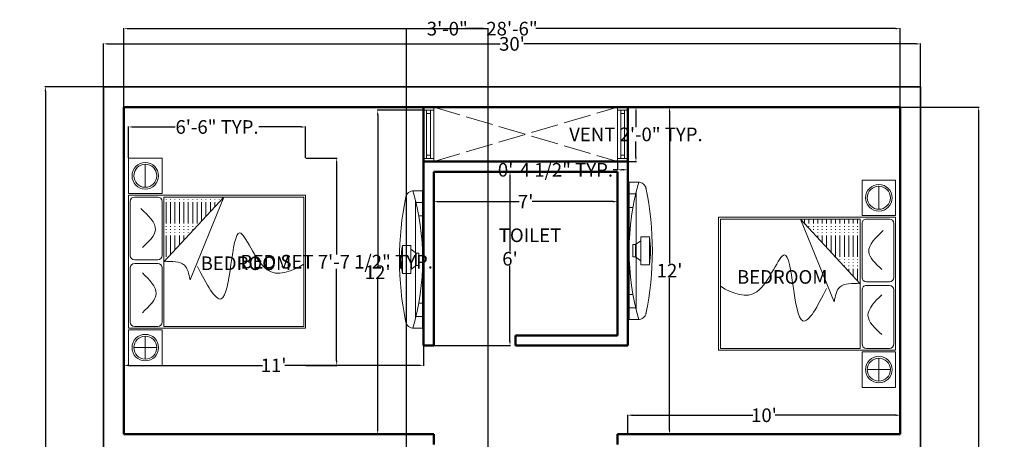
# Model space of a CAD drawing. Units: inches. Extents: x 134 to 568, y 15 to 554.
# Tile 7 of 7: x 134 to 568, y 369 to 554. Entities that reach past the tile are written whole.
import ezdxf

# ---------------------------------------------------------------- set-up
doc = ezdxf.new("R2010")
doc.units = ezdxf.units.IN
doc.header["$MEASUREMENT"] = 0
doc.linetypes.add('ACAD_ISO02W100', pattern=[15, 12, -3])
for name, color, linetype, lineweight in [('A-ANNO-DIMS', 2, 'Continuous', 18), ('A-AREA-IDEN', 7, 'Continuous', 25), ('A-EQPM', 8, 'Continuous', 18), ('A-FLOR-OPEN', 8, 'ACAD_ISO02W100', 18), ('A-FURN', 9, 'Continuous', 18), ('A-GLAZ', 4, 'Continuous', 18), ('A-WALL', 7, 'Continuous', 50), ('C-PROP', 7, 'Continuous', 35)]:
    doc.layers.add(name, color=color, linetype=linetype, lineweight=lineweight)
doc.styles.get("Standard").update_dxf_attribs({"font": 'arial.ttf'})
doc.dimstyles.get("Standard").update_dxf_attribs({"dimtxt": 6, "dimasz": 2, "dimexe": 0.18, "dimexo": 0.0625, "dimgap": 0.09, "dimtad": 0, "dimtih": 1, "dimtoh": 1, "dimdec": 0, "dimzin": 0, "dimdsep": 46, "dimlunit": 4, "dimtxsty": 'Standard', "dimcen": 0.09, "dimadec": 0, "dimazin": 0, "dimtfac": 1, "dimtdec": 0, "dimtofl": 0, "dimtmove": 0, "dimatfit": 3, "dimfxl": 1, "dimtolj": 1, "dimtzin": 0, "dimarcsym": 0})

# ---------------------------------------------------------------- blocks, each defined once
blk = doc.blocks.new('*D1')
at = {"layer": 'A-ANNO-DIMS', "color": 0, "lineweight": -2, "transparency": 16777216}
for p, q in [((171.08, 524.64), (171.08, 543.61)), ((173.08, 543.43), (345.9, 543.43)), ((529.08, 543.43), (356.26, 543.43)), ((531.08, 524.64), (531.08, 543.61))]:
    blk.add_line(p, q, dxfattribs=at)
at = {"layer": 'A-ANNO-DIMS', "color": 0, "transparency": 16777216}
for points in [[(173.08, 543.76), (173.08, 543.1), (171.08, 543.43)], [(529.08, 543.76), (529.08, 543.1), (531.08, 543.43)]]:
    blk.add_solid(points, dxfattribs=at)
at = {"layer": 'Defpoints', "color": 0, "transparency": 16777216}
for p in [(531.08, 543.43), (171.08, 524.58), (531.08, 524.58)]:
    blk.add_point(p, dxfattribs=at)
at = {"layer": 'A-ANNO-DIMS', "color": 0, "transparency": 16777216, "insert": (351.08, 543.43), "char_height": 6, "attachment_point": 5}
blk.add_mtext("\\A1;30'", dxfattribs=at)
blk = doc.blocks.new('*D16')
at = {"layer": 'A-ANNO-DIMS', "color": 0, "lineweight": -2, "transparency": 16777216}
for p, q in [((316.65, 487.08), (350.37, 487.08)), ((350.19, 485.08), (350.19, 451.99)), ((350.19, 412.58), (350.19, 445.68)), ((316.65, 410.58), (350.37, 410.58))]:
    blk.add_line(p, q, dxfattribs=at)
at = {"layer": 'A-ANNO-DIMS', "color": 0, "transparency": 16777216}
for points in [[(349.85, 485.08), (350.52, 485.08), (350.19, 487.08)], [(349.85, 412.58), (350.52, 412.58), (350.19, 410.58)]]:
    blk.add_solid(points, dxfattribs=at)
at = {"layer": 'Defpoints', "color": 0, "transparency": 16777216}
for p in [(316.58, 487.08), (316.58, 410.58), (350.19, 410.58)]:
    blk.add_point(p, dxfattribs=at)
at = {"layer": 'A-ANNO-DIMS', "color": 0, "transparency": 16777216, "insert": (350.19, 448.83), "char_height": 6, "attachment_point": 5}
blk.add_mtext("\\A1;6'", dxfattribs=at)
blk = doc.blocks.new('*D17')
at = {"layer": 'A-ANNO-DIMS', "color": 0, "lineweight": -2, "transparency": 16777216}
for p, q in [((316.58, 487.02), (316.58, 473.78)), ((397.58, 487.02), (397.58, 473.78)), ((318.58, 473.96), (354.26, 473.96)), ((395.58, 473.96), (359.91, 473.96))]:
    blk.add_line(p, q, dxfattribs=at)
at = {"layer": 'A-ANNO-DIMS', "color": 0, "transparency": 16777216}
for points in [[(318.58, 474.29), (318.58, 473.62), (316.58, 473.96)], [(395.58, 474.29), (395.58, 473.62), (397.58, 473.96)]]:
    blk.add_solid(points, dxfattribs=at)
at = {"layer": 'Defpoints', "color": 0, "transparency": 16777216}
for p in [(316.58, 487.08), (397.58, 487.08), (397.58, 473.96)]:
    blk.add_point(p, dxfattribs=at)
at = {"layer": 'A-ANNO-DIMS', "color": 0, "transparency": 16777216, "insert": (357.08, 473.96), "char_height": 6, "attachment_point": 5}
blk.add_mtext("\\A1;7'", dxfattribs=at)
blk = doc.blocks.new('*D18')
at = {"layer": 'A-ANNO-DIMS', "color": 0, "lineweight": -2, "transparency": 16777216}
for p, q in [((312.02, 514.18), (291.74, 514.18)), ((291.92, 512.18), (291.92, 445.98)), ((291.92, 373.58), (291.92, 439.78)), ((316.52, 371.58), (291.74, 371.58))]:
    blk.add_line(p, q, dxfattribs=at)
at = {"layer": 'A-ANNO-DIMS', "color": 0, "transparency": 16777216}
for points in [[(291.59, 512.18), (292.25, 512.18), (291.92, 514.18)], [(291.59, 373.58), (292.25, 373.58), (291.92, 371.58)]]:
    blk.add_solid(points, dxfattribs=at)
at = {"layer": 'Defpoints', "color": 0, "transparency": 16777216}
for p in [(312.08, 514.18), (291.92, 371.58), (316.58, 371.58)]:
    blk.add_point(p, dxfattribs=at)
at = {"layer": 'A-ANNO-DIMS', "color": 0, "transparency": 16777216, "insert": (291.92, 442.88), "char_height": 6, "attachment_point": 5}
blk.add_mtext("\\A1;12'", dxfattribs=at)
blk = doc.blocks.new('*D19')
at = {"layer": 'A-ANNO-DIMS', "color": 0, "lineweight": -2, "transparency": 16777216}
for p, q in [((312.08, 410.52), (312.08, 401.71)), ((180.08, 371.64), (180.08, 402.07)), ((182.08, 401.89), (241.18, 401.89)), ((310.08, 401.89), (250.98, 401.89))]:
    blk.add_line(p, q, dxfattribs=at)
at = {"layer": 'A-ANNO-DIMS', "color": 0, "transparency": 16777216}
for points in [[(182.08, 402.22), (182.08, 401.55), (180.08, 401.89)], [(310.08, 402.22), (310.08, 401.55), (312.08, 401.89)]]:
    blk.add_solid(points, dxfattribs=at)
at = {"layer": 'Defpoints', "color": 0, "transparency": 16777216}
for p in [(312.08, 410.58), (180.08, 401.89), (180.08, 371.58)]:
    blk.add_point(p, dxfattribs=at)
at = {"layer": 'A-ANNO-DIMS', "color": 0, "transparency": 16777216, "insert": (246.08, 401.89), "char_height": 6, "attachment_point": 5}
blk.add_mtext("\\A1;11'", dxfattribs=at)
blk = doc.blocks.new('*D20')
at = {"layer": 'A-ANNO-DIMS', "color": 0, "lineweight": -2, "transparency": 16777216}
for p, q in [((522.02, 515.58), (420.3, 515.58)), ((420.48, 513.58), (420.48, 446.68)), ((420.48, 373.58), (420.48, 440.48)), ((522.02, 371.58), (420.3, 371.58))]:
    blk.add_line(p, q, dxfattribs=at)
at = {"layer": 'A-ANNO-DIMS', "color": 0, "transparency": 16777216}
for points in [[(420.14, 513.58), (420.81, 513.58), (420.48, 515.58)], [(420.14, 373.58), (420.81, 373.58), (420.48, 371.58)]]:
    blk.add_solid(points, dxfattribs=at)
at = {"layer": 'Defpoints', "color": 0, "transparency": 16777216}
for p in [(420.48, 515.58), (522.08, 515.58), (522.08, 371.58)]:
    blk.add_point(p, dxfattribs=at)
at = {"layer": 'A-ANNO-DIMS', "color": 0, "transparency": 16777216, "insert": (420.48, 443.58), "char_height": 6, "attachment_point": 5}
blk.add_mtext("\\A1;12'", dxfattribs=at)
blk = doc.blocks.new('*D21')
at = {"layer": 'A-ANNO-DIMS', "color": 0, "lineweight": -2, "transparency": 16777216}
for p, q in [((402.08, 371.64), (402.08, 380.11)), ((404.08, 379.93), (457.18, 379.93)), ((520.08, 379.93), (466.98, 379.93)), ((522.08, 371.64), (522.08, 380.11))]:
    blk.add_line(p, q, dxfattribs=at)
at = {"layer": 'A-ANNO-DIMS', "color": 0, "transparency": 16777216}
for points in [[(404.08, 380.27), (404.08, 379.6), (402.08, 379.93)], [(520.08, 380.27), (520.08, 379.6), (522.08, 379.93)]]:
    blk.add_solid(points, dxfattribs=at)
at = {"layer": 'Defpoints', "color": 0, "transparency": 16777216}
for p in [(402.08, 379.93), (402.08, 371.58), (522.08, 371.58)]:
    blk.add_point(p, dxfattribs=at)
at = {"layer": 'A-ANNO-DIMS', "color": 0, "transparency": 16777216, "insert": (462.08, 379.93), "char_height": 6, "attachment_point": 5}
blk.add_mtext("\\A1;10'", dxfattribs=at)
blk = doc.blocks.new('dfghj')
h = blk.add_hatch()
h.set_pattern_fill('ACAD_ISO06W100', color=256, scale=0.54, style=0)
h.set_pattern_definition([(0, (-45.6593, 81.268), (0, 2.7), [12.96, -1.62, 0.27, -1.62, 0.27, -3.51]), (0, (-45.6593, 81.268), (0, 2.7), [-18.36, 0.27, -1.62])])
h.paths.add_polyline_path([(495.42, 683.37), (534.84, 646.9), (534.84, 683.37)])
for p, q in [((432.24, 704.97), (453.84, 704.97)), ((432.24, 704.97), (432.24, 684.45)), ((453.84, 704.97), (453.84, 684.45)), ((454.92, 704.97), (454.92, 596.97)), ((454.92, 704.97), (535.92, 704.97)), ((458.7, 703.89), (491.64, 703.89)), ((499.2, 703.89), (532.14, 703.89)), ((535.92, 704.97), (535.92, 596.97)), ((537, 704.97), (558.6, 704.97)), ((537, 704.97), (537, 684.45)), ((558.6, 704.97), (558.6, 684.45)), ((443.04, 701.73), (443.04, 687.69)), ((456, 701.19), (456, 687.15)), ((494.34, 701.19), (494.34, 687.15)), ((496.5, 701.19), (496.5, 687.15)), ((534.84, 701.19), (534.84, 687.15)), ((436.02, 694.71), (450.06, 694.71)), ((540.78, 694.71), (554.82, 694.71)), ((432.24, 684.45), (453.84, 684.45)), ((456, 683.37), (456, 598.05)), ((456, 683.37), (534.84, 683.37)), ((458.7, 684.45), (491.64, 684.45)), ((495.42, 683.37), (534.84, 646.9)), ((499.2, 684.45), (532.14, 684.45)), ((534.84, 683.37), (534.84, 598.05)), ((537, 684.45), (558.6, 684.45)), ((484.41, 667.43), (534.84, 646.9)), ((454.92, 596.97), (535.92, 596.97)), ((456, 598.05), (534.84, 598.05))]:
    blk.add_line(p, q)
for centre, radius in [((443.04, 694.71), 8.1), ((547.8, 694.71), 8.1), ((443.04, 694.71), 7.02), ((547.8, 694.71), 7.02)]:
    blk.add_circle(centre, radius)
for centre, start, end in [((458.7, 701.19), 90, 180), ((491.64, 701.19), 0, 90), ((499.2, 701.19), 90, 180), ((532.14, 701.19), 0, 90), ((458.7, 687.15), 180, 270), ((491.64, 687.15), 270, 0), ((499.2, 687.15), 180, 270), ((532.14, 687.15), 270, 0)]:
    blk.add_arc(centre, 2.7, start, end)
for points, knots in [([(504.09, 696.5), (507.65, 692.67), (515.42, 684.32), (523.53, 692.82), (527.93, 697.43)], [0, 0, 0, 0, 13.366336, 29.180825, 29.180825, 29.180825, 29.180825]), ([(464.35, 696.5), (468.22, 692.37), (476.17, 683.88), (484.43, 692.22), (488.66, 696.5)], [0, 0, 0, 0, 14.397067, 29.563029, 29.563029, 29.563029, 29.563029]), ([(484.41, 667.43), (487.91, 668.15), (496.06, 669.8), (495.65, 678.44), (495.42, 683.37)], [0, 0, 0, 0, 9.56516, 22.24155, 22.24155, 22.24155, 22.24155]), ([(492.4, 662.87), (481.85, 657.38), (453.25, 642.49), (538.24, 642.18), (482, 623.43), (489.25, 606.12), (493.82, 598.05)], [0, 0, 0, 0, 451.778418, 1224.724352, 1743.990777, 2173.853229, 2173.853229, 2173.853229, 2173.853229])]:
    blk.add_open_spline(points, degree=3, knots=knots)
blk = doc.blocks.new('A$C78AE5658')
for p, q in [((1515, 306), (1515, 524)), ((1515, 524), (2236, 524)), ((2236, 306), (2236, 524)), ((1515, 306), (2236, 306)), ((1613, 306), (1716, 168)), ((2137, 306), (2034, 168)), ((98, 250), (98, 252)), ((98, 250), (98, 0)), ((3648, 0), (98, 0)), ((348, 184), (3398, 184)), ((398, 0), (398, 172)), ((748, 0), (748, 99)), ((2034, 168), (1716, 168)), ((1716, 168), (1716, 98)), ((2034, 98), (1716, 98)), ((2034, 168), (2034, 98)), ((2998, 0), (2998, 99)), ((3348, 0), (3348, 172)), ((3648, 250), (3648, 252)), ((3648, 0), (3648, 250))]:
    blk.add_line(p, q)
blk.add_lwpolyline([(246, 432, -0.103184), (3500, 432, -0.103184)], format="xyb")
for centre, radius, start, end in [((1875, -1675), 2228, 80.6925, 99.3075), ((298, 239), 200, 98.4687, 183.693), ((3449, 239), 200, 356.307, 81.5313), ((1873, 6426), 6426, 253.9658, 286.0342)]:
    blk.add_arc(centre, radius, start, end)
blk = doc.blocks.new('WIN-24IN-VENT')
for p, q in [((0, 22.6), (4.5, 22.6)), ((1.4, 22.6), (1.4, 1.4)), ((3.1, 22.6), (3.1, 1.4)), ((4.5, 24), (4.5, 0)), ((1.4, 21.2), (3.1, 21.2)), ((0, 1.4), (4.5, 1.4)), ((1.4, 2.8), (3.1, 2.8))]:
    blk.add_line(p, q)
blk = doc.blocks.new('*D36')
at = {"layer": 'A-ANNO-DIMS', "color": 0, "lineweight": -2, "transparency": 16777216}
for p, q in [((260.21, 493.15), (274.02, 493.15)), ((273.84, 491.15), (273.84, 450.71)), ((273.84, 403.89), (273.84, 444.33)), ((260.21, 401.89), (274.02, 401.89))]:
    blk.add_line(p, q, dxfattribs=at)
at = {"layer": 'A-ANNO-DIMS', "color": 0, "transparency": 16777216}
for points in [[(273.51, 491.15), (274.17, 491.15), (273.84, 493.15)], [(273.51, 403.89), (274.17, 403.89), (273.84, 401.89)]]:
    blk.add_solid(points, dxfattribs=at)
at = {"layer": 'Defpoints', "color": 0, "transparency": 16777216}
for p in [(260.15, 493.15), (273.84, 493.15), (260.15, 401.89)]:
    blk.add_point(p, dxfattribs=at)
at = {"layer": 'A-ANNO-DIMS', "color": 0, "transparency": 16777216, "insert": (273.84, 447.52), "char_height": 6, "attachment_point": 5}
blk.add_mtext('\\A1;BED SET 7\'-7 1/2" TYP.', dxfattribs=at)
blk = doc.blocks.new('*D37')
at = {"layer": 'A-ANNO-DIMS', "color": 0, "lineweight": -2, "transparency": 16777216}
for p, q in [((182.14, 493.22), (182.14, 507.02)), ((184.14, 506.84), (202.75, 506.84)), ((258.15, 506.84), (239.54, 506.84)), ((260.15, 493.22), (260.15, 507.02))]:
    blk.add_line(p, q, dxfattribs=at)
at = {"layer": 'A-ANNO-DIMS', "color": 0, "transparency": 16777216}
for points in [[(184.14, 507.18), (184.14, 506.51), (182.14, 506.84)], [(258.15, 507.18), (258.15, 506.51), (260.15, 506.84)]]:
    blk.add_solid(points, dxfattribs=at)
at = {"layer": 'Defpoints', "color": 0, "transparency": 16777216}
for p in [(182.14, 506.84), (182.14, 493.15), (260.15, 493.15)]:
    blk.add_point(p, dxfattribs=at)
at = {"layer": 'A-ANNO-DIMS', "color": 0, "transparency": 16777216, "insert": (221.15, 506.84), "char_height": 6, "attachment_point": 5}
blk.add_mtext('\\A1;6\'-6" TYP.', dxfattribs=at)
blk = doc.blocks.new('*D54')
at = {"layer": 'A-ANNO-DIMS', "color": 0, "lineweight": -2, "transparency": 16777216}
for p, q in [((402.15, 515.58), (405.86, 515.58)), ((405.68, 513.58), (405.68, 506.74)), ((405.68, 493.58), (405.68, 500.43)), ((402.15, 491.58), (405.86, 491.58))]:
    blk.add_line(p, q, dxfattribs=at)
at = {"layer": 'A-ANNO-DIMS', "color": 0, "transparency": 16777216}
for points in [[(405.35, 513.58), (406.02, 513.58), (405.68, 515.58)], [(405.35, 493.58), (406.02, 493.58), (405.68, 491.58)]]:
    blk.add_solid(points, dxfattribs=at)
at = {"layer": 'Defpoints', "color": 0, "transparency": 16777216}
for p in [(402.08, 515.58), (402.08, 491.58), (405.68, 491.58)]:
    blk.add_point(p, dxfattribs=at)
at = {"layer": 'A-ANNO-DIMS', "color": 0, "transparency": 16777216, "insert": (405.68, 503.58), "char_height": 6, "attachment_point": 5}
blk.add_mtext('\\A1;VENT 2\'-0" TYP.', dxfattribs=at)
blk = doc.blocks.new('*D55')
at = {"layer": 'A-ANNO-DIMS', "color": 0, "lineweight": -2, "transparency": 16777216}
for p, q in [((397.58, 491.52), (397.58, 487.8)), ((402.08, 491.52), (402.08, 487.8)), ((397.58, 487.98), (395.58, 487.98)), ((400.08, 487.98), (399.58, 487.98))]:
    blk.add_line(p, q, dxfattribs=at)
at = {"layer": 'A-ANNO-DIMS', "color": 0, "transparency": 16777216}
for points in [[(399.58, 488.32), (399.58, 487.65), (397.58, 487.98)], [(400.08, 488.32), (400.08, 487.65), (402.08, 487.98)]]:
    blk.add_solid(points, dxfattribs=at)
at = {"layer": 'Defpoints', "color": 0, "transparency": 16777216}
for p in [(397.58, 491.58), (402.08, 491.58), (397.58, 487.98)]:
    blk.add_point(p, dxfattribs=at)
at = {"layer": 'A-ANNO-DIMS', "color": 0, "transparency": 16777216, "insert": (370.22, 487.98), "char_height": 6, "attachment_point": 5}
blk.add_mtext('\\A1;0\'-4 1/2" TYP.', dxfattribs=at)
blk = doc.blocks.new('*D58')
at = {"layer": 'A-ANNO-DIMS', "color": 0, "lineweight": -2, "transparency": 16777216}
for p, q in [((171.02, 524.58), (145.35, 524.58)), ((145.53, 522.58), (145.53, 287.74)), ((145.53, 46.58), (145.53, 281.43)), ((171.02, 44.58), (145.35, 44.58))]:
    blk.add_line(p, q, dxfattribs=at)
at = {"layer": 'A-ANNO-DIMS', "color": 0, "transparency": 16777216}
for points in [[(145.2, 522.58), (145.87, 522.58), (145.53, 524.58)], [(145.2, 46.58), (145.87, 46.58), (145.53, 44.58)]]:
    blk.add_solid(points, dxfattribs=at)
at = {"layer": 'Defpoints', "color": 0, "transparency": 16777216}
for p in [(145.53, 524.58), (171.08, 524.58), (171.08, 44.58)]:
    blk.add_point(p, dxfattribs=at)
at = {"layer": 'A-ANNO-DIMS', "color": 0, "transparency": 16777216, "insert": (145.53, 284.58), "char_height": 6, "attachment_point": 5}
blk.add_mtext('\\A1;40\'-0"', dxfattribs=at)
blk = doc.blocks.new('*D59')
at = {"layer": 'A-ANNO-DIMS', "color": 0, "lineweight": -2, "transparency": 16777216}
for p, q in [((180.08, 515.64), (180.08, 550.31)), ((182.08, 550.13), (340.64, 550.13)), ((520.08, 550.13), (361.53, 550.13)), ((522.08, 515.64), (522.08, 550.31))]:
    blk.add_line(p, q, dxfattribs=at)
at = {"layer": 'A-ANNO-DIMS', "color": 0, "transparency": 16777216}
for points in [[(182.08, 550.47), (182.08, 549.8), (180.08, 550.13)], [(520.08, 550.47), (520.08, 549.8), (522.08, 550.13)]]:
    blk.add_solid(points, dxfattribs=at)
at = {"layer": 'Defpoints', "color": 0, "transparency": 16777216}
for p in [(522.08, 550.13), (180.08, 515.58), (522.08, 515.58)]:
    blk.add_point(p, dxfattribs=at)
at = {"layer": 'A-ANNO-DIMS', "color": 0, "transparency": 16777216, "insert": (351.08, 550.13), "char_height": 6, "attachment_point": 5}
blk.add_mtext('\\A1;28\'-6"', dxfattribs=at)
blk = doc.blocks.new('*D60')
at = {"layer": 'A-ANNO-DIMS', "color": 0, "lineweight": -2, "transparency": 16777216}
for p, q in [((522.15, 515.58), (556.81, 515.58)), ((556.63, 513.58), (556.63, 283.24)), ((556.63, 46.58), (556.63, 276.93)), ((522.15, 44.58), (556.81, 44.58))]:
    blk.add_line(p, q, dxfattribs=at)
at = {"layer": 'A-ANNO-DIMS', "color": 0, "transparency": 16777216}
for points in [[(556.3, 513.58), (556.97, 513.58), (556.63, 515.58)], [(556.3, 46.58), (556.97, 46.58), (556.63, 44.58)]]:
    blk.add_solid(points, dxfattribs=at)
at = {"layer": 'Defpoints', "color": 0, "transparency": 16777216}
for p in [(522.08, 515.58), (556.63, 515.58), (522.08, 44.58)]:
    blk.add_point(p, dxfattribs=at)
at = {"layer": 'A-ANNO-DIMS', "color": 0, "transparency": 16777216, "insert": (556.63, 280.08), "char_height": 6, "attachment_point": 5}
blk.add_mtext('\\A1;39\'-3"', dxfattribs=at)
blk = doc.blocks.new('*D63')
at = {"layer": 'A-ANNO-DIMS', "color": 0, "lineweight": -2, "transparency": 16777216}
for p, q in [((304.58, 114.64), (304.58, 550.31)), ((306.58, 550.13), (314.52, 550.13)), ((338.58, 550.13), (330.65, 550.13)), ((340.58, 114.64), (340.58, 550.31))]:
    blk.add_line(p, q, dxfattribs=at)
at = {"layer": 'A-ANNO-DIMS', "color": 0, "transparency": 16777216}
for points in [[(306.58, 550.47), (306.58, 549.8), (304.58, 550.13)], [(338.58, 550.47), (338.58, 549.8), (340.58, 550.13)]]:
    blk.add_solid(points, dxfattribs=at)
at = {"layer": 'Defpoints', "color": 0, "transparency": 16777216}
for p in [(340.58, 550.13), (304.58, 114.58), (340.58, 114.58)]:
    blk.add_point(p, dxfattribs=at)
at = {"layer": 'A-ANNO-DIMS', "color": 0, "transparency": 16777216, "insert": (322.58, 550.13), "char_height": 6, "attachment_point": 5}
blk.add_mtext('\\A1;3\'-0"', dxfattribs=at)

msp = doc.modelspace()

# ---------------------------------------------------------------- linework, layer by layer
at = {"layer": 'A-FLOR-OPEN'}
for p, q in [((316.58, 491.58), (397.58, 515.58)), ((316.58, 515.58), (397.58, 491.58))]:
    msp.add_line(p, q, dxfattribs=at)
at = {"layer": 'A-WALL'}
for p, q in [((180.08, 515.58), (312.08, 515.58)), ((180.08, 515.58), (180.08, 371.58)), ((312.08, 515.58), (312.08, 410.58)), ((312.08, 515.58), (402.08, 515.58)), ((402.08, 410.58), (402.08, 515.58)), ((402.08, 515.58), (522.08, 515.58)), ((522.08, 371.58), (522.08, 515.58)), ((312.08, 491.58), (402.08, 491.58)), ((316.58, 487.08), (397.58, 487.08)), ((316.58, 487.08), (316.58, 410.58)), ((397.58, 415.08), (397.58, 487.08)), ((352.58, 415.08), (397.58, 415.08)), ((352.58, 415.08), (352.58, 410.58)), ((312.08, 410.58), (316.58, 410.58)), ((352.58, 410.58), (402.08, 410.58)), ((180.08, 371.58), (316.58, 371.58)), ((316.58, 371.58), (316.58, 367.08)), ((397.58, 367.08), (397.58, 371.58)), ((397.58, 371.58), (522.08, 371.58))]:
    msp.add_line(p, q, dxfattribs=at)
at = {"layer": 'C-PROP'}
for p, q in [((171.08, 524.58), (531.08, 524.58)), ((171.08, 524.58), (171.08, 44.58)), ((531.08, 44.58), (531.08, 524.58))]:
    msp.add_line(p, q, dxfattribs=at)

# ---------------------------------------------------------------- block references
at = {"layer": 'A-EQPM', "yscale": 0.0170389131376971, "zscale": 0.0170389131376971}
for p, xscale, rotation in [((402.69, 420.37), -0.0170389131376971, 270), ((311.73, 416.57), 0.0170389131376971, 90)]:
    msp.add_blockref('A$C78AE5658', p, dxfattribs=dict(at, xscale=xscale, rotation=rotation))
at = {"layer": 'A-FURN', "yscale": 0.7222806032890517, "zscale": 0.7222806032890517}
for p, xscale, rotation in [((691.33, 89.69), 0.7222806032890517, 90), ((10.9, 80.01), -0.7222806032890517, 270)]:
    msp.add_blockref('dfghj', p, dxfattribs=dict(at, xscale=xscale, rotation=rotation))
at = {"layer": 'A-GLAZ'}
msp.add_blockref('WIN-24IN-VENT', (312.08, 491.58), dxfattribs=at)
at = {"layer": 'A-GLAZ', "rotation": 180}
msp.add_blockref('WIN-24IN-VENT', (402.08, 515.58), dxfattribs=at)

# ---------------------------------------------------------------- texts
at = {"layer": 'A-AREA-IDEN', "char_height": 6, "attachment_point": 1}
for s, width, insert in [('\\pxqc;TOILET', 65.8409, (326.11, 462.18)), ('BEDROOM', 59.5758, (213.94, 449.83)), ('BEDROOM', 59.5758, (450.19, 443.82))]:
    msp.add_mtext_dynamic_manual_height_columns(s, width=width, gutter_width=30, heights=[0], dxfattribs=dict(at, insert=insert))

# ---------------------------------------------------------------- dimensions: what is measured, and where the dimension line sits
at = {"layer": 'A-ANNO-DIMS'}
for base, p1, p2, override, picture, middle in [((522.08, 550.13), (180.08, 515.58), (522.08, 515.58), {"dimdec": 1, "dimlfac": 1, "dimrnd": 0, "dimzin": 1, "dimdsep": 46, "dimlunit": 4, "dimfrac": 2}, '*D59', (351.08, 550.13)), ((340.58, 550.13), (304.58, 114.58), (340.58, 114.58), {"dimdec": 1, "dimlfac": 1, "dimrnd": 0, "dimzin": 1, "dimdsep": 46, "dimlunit": 4, "dimfrac": 2}, '*D63', (322.58, 550.13)), ((531.08, 543.43), (171.08, 524.58), (531.08, 524.58), {"dimclrd": 0, "dimclre": 0, "dimclrt": 0}, '*D1', (351.08, 543.43)), ((180.08, 401.89), (312.08, 410.58), (180.08, 371.58), {"dimclrd": 0, "dimclre": 0, "dimclrt": 0}, '*D19', (246.08, 401.89)), ((402.08, 379.93), (522.08, 371.58), (402.08, 371.58), {"dimclrd": 0, "dimclre": 0, "dimclrt": 0}, '*D21', (462.08, 379.93))]:
    dim = msp.add_linear_dim(base=base, p1=p1, p2=p2, dimstyle='Standard', override=override, dxfattribs=at)
    dim.commit()
    dim.dimension.update_dxf_attribs({"geometry": picture, "text_midpoint": middle})
for base, p1, p2, override, picture, middle in [((145.53, 524.58), (171.08, 44.58), (171.08, 524.58), {"dimdec": 1, "dimlfac": 1, "dimrnd": 0, "dimzin": 1, "dimdsep": 46, "dimlunit": 4, "dimfrac": 2}, '*D58', (145.53, 284.58)), ((420.48, 515.58), (522.08, 371.58), (522.08, 515.58), {"dimclrd": 0, "dimclre": 0, "dimclrt": 0}, '*D20', (420.48, 443.58)), ((556.63, 515.58), (522.08, 44.58), (522.08, 515.58), {"dimdec": 1, "dimlfac": 1, "dimrnd": 0, "dimzin": 1, "dimdsep": 46, "dimlunit": 4, "dimfrac": 2}, '*D60', (556.63, 280.08))]:
    dim = msp.add_linear_dim(base=base, p1=p1, p2=p2, angle=90, dimstyle='Standard', override=override, dxfattribs=at)
    dim.commit()
    dim.dimension.update_dxf_attribs({"geometry": picture, "text_midpoint": middle})
for base, p1, p2, angle, text, override, picture, middle in [((405.68, 491.58), (402.08, 515.58), (402.08, 491.58), 270, 'VENT <> TYP.', {"dimdec": 1, "dimlfac": 1, "dimrnd": 0, "dimzin": 1, "dimdsep": 46, "dimlunit": 4, "dimfrac": 2}, '*D54', (405.68, 503.58)), ((182.14, 506.84), (260.15, 493.15), (182.14, 493.15), 180, '<> TYP.', {"dimdec": 1, "dimlfac": 1, "dimrnd": 0, "dimzin": 1, "dimdsep": 46, "dimlunit": 4, "dimfrac": 2}, '*D37', (221.15, 506.84)), ((291.92, 371.58), (312.08, 514.18), (316.58, 371.58), 90, "12'", {"dimclrd": 0, "dimclre": 0, "dimclrt": 0}, '*D18', (291.92, 442.88)), ((397.58, 487.98), (402.08, 491.58), (397.58, 491.58), 180, '<> TYP.', {"dimdec": 1, "dimlfac": 1, "dimrnd": 0, "dimzin": 1, "dimdsep": 46, "dimlunit": 4, "dimfrac": 2}, '*D55', (370.22, 487.98)), ((273.84, 493.15), (260.15, 401.89), (260.15, 493.15), 90, 'BED SET <> TYP.', {"dimdec": 1, "dimlfac": 1, "dimrnd": 0, "dimzin": 1, "dimdsep": 46, "dimlunit": 4, "dimfrac": 2}, '*D36', (273.84, 447.52)), ((350.19, 410.58), (316.58, 487.08), (316.58, 410.58), 90, "6'", {"dimclrd": 0, "dimclre": 0, "dimclrt": 0}, '*D16', (350.19, 448.83))]:
    dim = msp.add_linear_dim(base=base, p1=p1, p2=p2, angle=angle, text=text, dimstyle='Standard', override=override, dxfattribs=at)
    dim.commit()
    dim.dimension.update_dxf_attribs({"geometry": picture, "text_midpoint": middle})
dim = msp.add_linear_dim(base=(397.58, 473.96), p1=(316.58, 487.08), p2=(397.58, 487.08), text="7'", dimstyle='Standard', override={"dimclrd": 0, "dimclre": 0, "dimclrt": 0}, dxfattribs=at)
dim.commit()
dim.dimension.update_dxf_attribs({"geometry": '*D17', "text_midpoint": (357.08, 473.96)})

doc.saveas('drawing.dxf')
